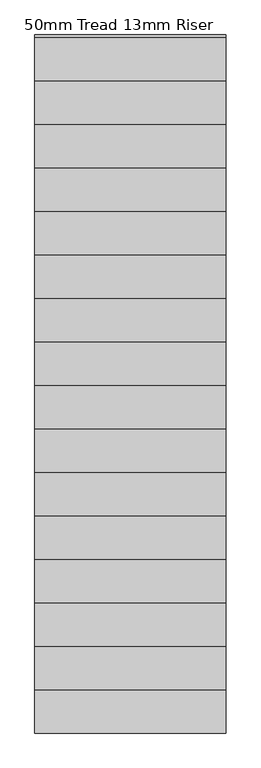
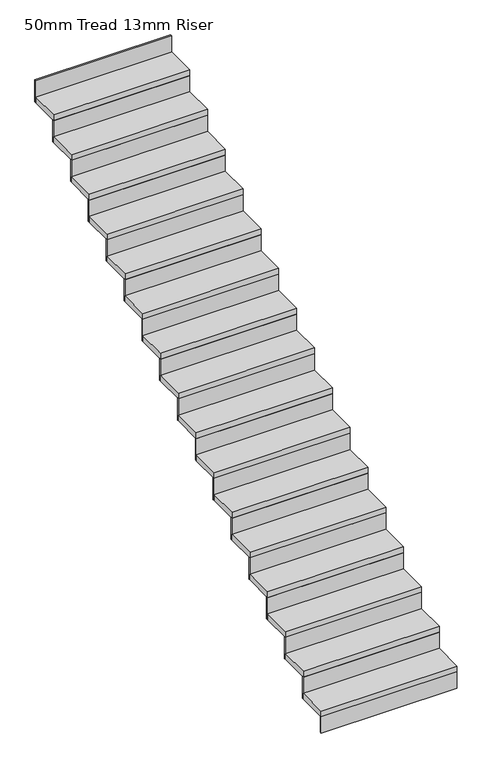
"""IFC4 building model written with IfcOpenShell, lengths in millimetres: stair flight geometry, 50mm Tread 13mm Riser."""

from ifc_helpers import new_model, si_unit, frame, origin, origin_with_axes, place, context, project, spatial, polyline, outline, extrude, source, transform, mapped, element, save


def stair_flight_50mm_tread_13mm_riser_6fdf431e(model_context):
    return source(origin(), model_context, "Body", "SweptSolid", [
        extrude(outline(polyline([(-3919.0317552, -2754.2477501), (-3919.0317552, -2766.7477501), (-5019.0317552, -2766.7477501), (-5019.0317552, -2754.2477501), (-3919.0317552, -2754.2477501)])), origin_with_axes(), (0.0, 0.0, 1.0), 138.2352941),
        extrude(outline(polyline([(-5019.0317552, -2516.7477501), (-3919.0317552, -2516.7477501), (-3919.0317552, -2766.7477501), (-5019.0317552, -2766.7477501), (-5019.0317552, -2516.7477501)])), frame((0.0, 0.0, 138.2352941), z_axis=(0.0, 0.0, 1.0), x_axis=(1.0, 0.0, 0.0)), (0.0, 0.0, 1.0), 50.0),
        extrude(outline(polyline([(-3919.0317552, -2504.2477501), (-3919.0317552, -2516.7477501), (-5019.0317552, -2516.7477501), (-5019.0317552, -2504.2477501), (-3919.0317552, -2504.2477501)])), frame((0.0, 0.0, 138.2352941), z_axis=(0.0, 0.0, 1.0), x_axis=(1.0, 0.0, 0.0)), (0.0, 0.0, 1.0), 188.2352941),
        extrude(outline(polyline([(-5019.0317552, -2266.7477501), (-3919.0317552, -2266.7477501), (-3919.0317552, -2516.7477501), (-5019.0317552, -2516.7477501), (-5019.0317552, -2266.7477501)])), frame((0.0, 0.0, 326.4705882), z_axis=(0.0, 0.0, 1.0), x_axis=(1.0, 0.0, 0.0)), (0.0, 0.0, 1.0), 50.0),
        extrude(outline(polyline([(-3919.0317552, -2254.2477501), (-3919.0317552, -2266.7477501), (-5019.0317552, -2266.7477501), (-5019.0317552, -2254.2477501), (-3919.0317552, -2254.2477501)])), frame((0.0, 0.0, 326.4705882), z_axis=(0.0, 0.0, 1.0), x_axis=(1.0, 0.0, 0.0)), (0.0, 0.0, 1.0), 188.2352941),
        extrude(outline(polyline([(-5019.0317552, -2016.7477501), (-3919.0317552, -2016.7477501), (-3919.0317552, -2266.7477501), (-5019.0317552, -2266.7477501), (-5019.0317552, -2016.7477501)])), frame((0.0, 0.0, 514.7058824), z_axis=(0.0, 0.0, 1.0), x_axis=(1.0, 0.0, 0.0)), (0.0, 0.0, 1.0), 50.0),
        extrude(outline(polyline([(-3919.0317552, -2004.2477501), (-3919.0317552, -2016.7477501), (-5019.0317552, -2016.7477501), (-5019.0317552, -2004.2477501), (-3919.0317552, -2004.2477501)])), frame((0.0, 0.0, 514.7058824), z_axis=(0.0, 0.0, 1.0), x_axis=(1.0, 0.0, 0.0)), (0.0, 0.0, 1.0), 188.2352941),
        extrude(outline(polyline([(-5019.0317552, -1766.7477501), (-3919.0317552, -1766.7477501), (-3919.0317552, -2016.7477501), (-5019.0317552, -2016.7477501), (-5019.0317552, -1766.7477501)])), frame((0.0, 0.0, 702.9411765), z_axis=(0.0, 0.0, 1.0), x_axis=(1.0, 0.0, 0.0)), (0.0, 0.0, 1.0), 50.0),
        extrude(outline(polyline([(-3919.0317552, -1754.2477501), (-3919.0317552, -1766.7477501), (-5019.0317552, -1766.7477501), (-5019.0317552, -1754.2477501), (-3919.0317552, -1754.2477501)])), frame((0.0, 0.0, 702.9411765), z_axis=(0.0, 0.0, 1.0), x_axis=(1.0, 0.0, 0.0)), (0.0, 0.0, 1.0), 188.2352941),
        extrude(outline(polyline([(-5019.0317552, -1516.7477501), (-3919.0317552, -1516.7477501), (-3919.0317552, -1766.7477501), (-5019.0317552, -1766.7477501), (-5019.0317552, -1516.7477501)])), frame((0.0, 0.0, 891.1764706), z_axis=(0.0, 0.0, 1.0), x_axis=(1.0, 0.0, 0.0)), (0.0, 0.0, 1.0), 50.0),
        extrude(outline(polyline([(-3919.0317552, -1504.2477501), (-3919.0317552, -1516.7477501), (-5019.0317552, -1516.7477501), (-5019.0317552, -1504.2477501), (-3919.0317552, -1504.2477501)])), frame((0.0, 0.0, 891.1764706), z_axis=(0.0, 0.0, 1.0), x_axis=(1.0, 0.0, 0.0)), (0.0, 0.0, 1.0), 188.2352941),
        extrude(outline(polyline([(-5019.0317552, -1266.7477501), (-3919.0317552, -1266.7477501), (-3919.0317552, -1516.7477501), (-5019.0317552, -1516.7477501), (-5019.0317552, -1266.7477501)])), frame((0.0, 0.0, 1079.4117647), z_axis=(0.0, 0.0, 1.0), x_axis=(1.0, 0.0, 0.0)), (0.0, 0.0, 1.0), 50.0),
        extrude(outline(polyline([(-3919.0317552, -1254.2477501), (-3919.0317552, -1266.7477501), (-5019.0317552, -1266.7477501), (-5019.0317552, -1254.2477501), (-3919.0317552, -1254.2477501)])), frame((0.0, 0.0, 1079.4117647), z_axis=(0.0, 0.0, 1.0), x_axis=(1.0, 0.0, 0.0)), (0.0, 0.0, 1.0), 188.2352941),
        extrude(outline(polyline([(-5019.0317552, -1016.7477501), (-3919.0317552, -1016.7477501), (-3919.0317552, -1266.7477501), (-5019.0317552, -1266.7477501), (-5019.0317552, -1016.7477501)])), frame((0.0, 0.0, 1267.6470588), z_axis=(0.0, 0.0, 1.0), x_axis=(1.0, 0.0, 0.0)), (0.0, 0.0, 1.0), 50.0),
        extrude(outline(polyline([(-3919.0317552, -1004.2477501), (-3919.0317552, -1016.7477501), (-5019.0317552, -1016.7477501), (-5019.0317552, -1004.2477501), (-3919.0317552, -1004.2477501)])), frame((0.0, 0.0, 1267.6470588), z_axis=(0.0, 0.0, 1.0), x_axis=(1.0, 0.0, 0.0)), (0.0, 0.0, 1.0), 188.2352941),
        extrude(outline(polyline([(-5019.0317552, -766.7477501), (-3919.0317552, -766.7477501), (-3919.0317552, -1016.7477501), (-5019.0317552, -1016.7477501), (-5019.0317552, -766.7477501)])), frame((0.0, 0.0, 1455.8823529), z_axis=(0.0, 0.0, 1.0), x_axis=(1.0, 0.0, 0.0)), (0.0, 0.0, 1.0), 50.0),
        extrude(outline(polyline([(-3919.0317552, -754.2477501), (-3919.0317552, -766.7477501), (-5019.0317552, -766.7477501), (-5019.0317552, -754.2477501), (-3919.0317552, -754.2477501)])), frame((0.0, 0.0, 1455.8823529), z_axis=(0.0, 0.0, 1.0), x_axis=(1.0, 0.0, 0.0)), (0.0, 0.0, 1.0), 188.2352941),
        extrude(outline(polyline([(-5019.0317552, -516.7477501), (-3919.0317552, -516.7477501), (-3919.0317552, -766.7477501), (-5019.0317552, -766.7477501), (-5019.0317552, -516.7477501)])), frame((0.0, 0.0, 1644.1176471), z_axis=(0.0, 0.0, 1.0), x_axis=(1.0, 0.0, 0.0)), (0.0, 0.0, 1.0), 50.0),
        extrude(outline(polyline([(-3919.0317552, -504.2477501), (-3919.0317552, -516.7477501), (-5019.0317552, -516.7477501), (-5019.0317552, -504.2477501), (-3919.0317552, -504.2477501)])), frame((0.0, 0.0, 1644.1176471), z_axis=(0.0, 0.0, 1.0), x_axis=(1.0, 0.0, 0.0)), (0.0, 0.0, 1.0), 188.2352941),
        extrude(outline(polyline([(-5019.0317552, -266.7477501), (-3919.0317552, -266.7477501), (-3919.0317552, -516.7477501), (-5019.0317552, -516.7477501), (-5019.0317552, -266.7477501)])), frame((0.0, 0.0, 1832.3529412), z_axis=(0.0, 0.0, 1.0), x_axis=(1.0, 0.0, 0.0)), (0.0, 0.0, 1.0), 50.0),
        extrude(outline(polyline([(-3919.0317552, -254.2477501), (-3919.0317552, -266.7477501), (-5019.0317552, -266.7477501), (-5019.0317552, -254.2477501), (-3919.0317552, -254.2477501)])), frame((0.0, 0.0, 1832.3529412), z_axis=(0.0, 0.0, 1.0), x_axis=(1.0, 0.0, 0.0)), (0.0, 0.0, 1.0), 188.2352941),
        extrude(outline(polyline([(-5019.0317552, -16.7477501), (-3919.0317552, -16.7477501), (-3919.0317552, -266.7477501), (-5019.0317552, -266.7477501), (-5019.0317552, -16.7477501)])), frame((0.0, 0.0, 2020.5882353), z_axis=(0.0, 0.0, 1.0), x_axis=(1.0, 0.0, 0.0)), (0.0, 0.0, 1.0), 50.0),
        extrude(outline(polyline([(-3919.0317552, -4.2477501), (-3919.0317552, -16.7477501), (-5019.0317552, -16.7477501), (-5019.0317552, -4.2477501), (-3919.0317552, -4.2477501)])), frame((0.0, 0.0, 2020.5882353), z_axis=(0.0, 0.0, 1.0), x_axis=(1.0, 0.0, 0.0)), (0.0, 0.0, 1.0), 188.2352941),
        extrude(outline(polyline([(-5019.0317552, 233.2522499), (-3919.0317552, 233.2522499), (-3919.0317552, -16.7477501), (-5019.0317552, -16.7477501), (-5019.0317552, 233.2522499)])), frame((0.0, 0.0, 2208.8235294), z_axis=(0.0, 0.0, 1.0), x_axis=(1.0, 0.0, 0.0)), (0.0, 0.0, 1.0), 50.0),
        extrude(outline(polyline([(-3919.0317552, 245.7522499), (-3919.0317552, 233.2522499), (-5019.0317552, 233.2522499), (-5019.0317552, 245.7522499), (-3919.0317552, 245.7522499)])), frame((0.0, 0.0, 2208.8235294), z_axis=(0.0, 0.0, 1.0), x_axis=(1.0, 0.0, 0.0)), (0.0, 0.0, 1.0), 188.2352941),
        extrude(outline(polyline([(-5019.0317552, 483.2522499), (-3919.0317552, 483.2522499), (-3919.0317552, 233.2522499), (-5019.0317552, 233.2522499), (-5019.0317552, 483.2522499)])), frame((0.0, 0.0, 2397.0588235), z_axis=(0.0, 0.0, 1.0), x_axis=(1.0, 0.0, 0.0)), (0.0, 0.0, 1.0), 50.0),
        extrude(outline(polyline([(-3919.0317552, 495.7522499), (-3919.0317552, 483.2522499), (-5019.0317552, 483.2522499), (-5019.0317552, 495.7522499), (-3919.0317552, 495.7522499)])), frame((0.0, 0.0, 2397.0588235), z_axis=(0.0, 0.0, 1.0), x_axis=(1.0, 0.0, 0.0)), (0.0, 0.0, 1.0), 188.2352941),
        extrude(outline(polyline([(-5019.0317552, 733.2522499), (-3919.0317552, 733.2522499), (-3919.0317552, 483.2522499), (-5019.0317552, 483.2522499), (-5019.0317552, 733.2522499)])), frame((0.0, 0.0, 2585.2941176), z_axis=(0.0, 0.0, 1.0), x_axis=(1.0, 0.0, 0.0)), (0.0, 0.0, 1.0), 50.0),
        extrude(outline(polyline([(-3919.0317552, 745.7522499), (-3919.0317552, 733.2522499), (-5019.0317552, 733.2522499), (-5019.0317552, 745.7522499), (-3919.0317552, 745.7522499)])), frame((0.0, 0.0, 2585.2941176), z_axis=(0.0, 0.0, 1.0), x_axis=(1.0, 0.0, 0.0)), (0.0, 0.0, 1.0), 188.2352941),
        extrude(outline(polyline([(-5019.0317552, 983.2522499), (-3919.0317552, 983.2522499), (-3919.0317552, 733.2522499), (-5019.0317552, 733.2522499), (-5019.0317552, 983.2522499)])), frame((0.0, 0.0, 2773.5294118), z_axis=(0.0, 0.0, 1.0), x_axis=(1.0, 0.0, 0.0)), (0.0, 0.0, 1.0), 50.0),
        extrude(outline(polyline([(-3919.0317552, 995.7522499), (-3919.0317552, 983.2522499), (-5019.0317552, 983.2522499), (-5019.0317552, 995.7522499), (-3919.0317552, 995.7522499)])), frame((0.0, 0.0, 2773.5294118), z_axis=(0.0, 0.0, 1.0), x_axis=(1.0, 0.0, 0.0)), (0.0, 0.0, 1.0), 188.2352941),
        extrude(outline(polyline([(-3919.0317552, 1245.7522499), (-3919.0317552, 1233.2522499), (-5019.0317552, 1233.2522499), (-5019.0317552, 1245.7522499), (-3919.0317552, 1245.7522499)])), frame((0.0, 0.0, 2961.7647059), z_axis=(0.0, 0.0, 1.0), x_axis=(1.0, 0.0, 0.0)), (0.0, 0.0, 1.0), 188.2352941),
        extrude(outline(polyline([(-5019.0317552, 1233.2522499), (-3919.0317552, 1233.2522499), (-3919.0317552, 983.2522499), (-5019.0317552, 983.2522499), (-5019.0317552, 1233.2522499)])), frame((0.0, 0.0, 2961.7647059), z_axis=(0.0, 0.0, 1.0), x_axis=(1.0, 0.0, 0.0)), (0.0, 0.0, 1.0), 50.0),
    ])


if __name__ == "__main__":
    model = new_model("IFC4")
    model_context = context("Model", 3, world=origin())
    ifc_project = project(units=[si_unit("LENGTHUNIT", "METRE", prefix="MILLI")], contexts=[model_context])
    site = spatial("IfcSite", under=ifc_project)
    building = spatial("IfcBuilding", under=site)
    placement = place(None, origin())
    stair_flight_50mm_tread_13mm_riser_shape = stair_flight_50mm_tread_13mm_riser_6fdf431e(model_context)
    element("IfcStairFlight", 1, ObjectType="50mm Tread 13mm Riser", at=placement, inside=building, context=model_context, shape_type="MappedRepresentation", body=[
        mapped(stair_flight_50mm_tread_13mm_riser_shape, transform((0.0, 0.0, 0.0), x_axis=(1.0, 0.0, 0.0), y_axis=(0.0, 1.0, 0.0), z_axis=(0.0, 0.0, 1.0))),
    ])
    save(model, "model.ifc")
